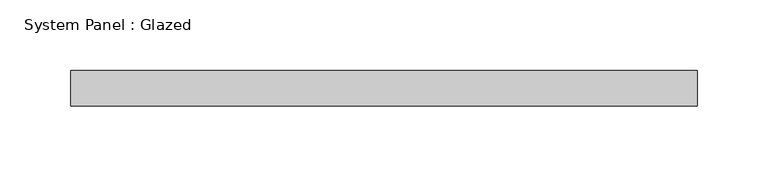
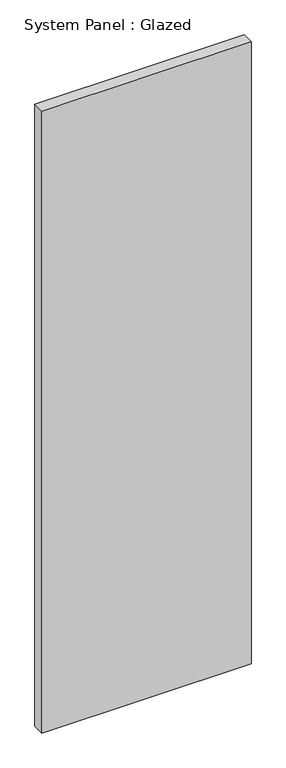
"""IFC4 building model written with IfcOpenShell, lengths in millimetres: plate geometry, System Panel : Glazed."""

from ifc_helpers import new_model, si_unit, origin, origin_with_axes, place, context, project, spatial, polyline, outline, extrude, source, transform, mapped, element, save


def system_panel_glazed_17c4a998(model_context):
    return source(origin(), model_context, "Body", "SweptSolid", [
        extrude(outline(polyline([(222.25, 19.05), (-222.25, 19.05), (-222.25, 44.45), (222.25, 44.45), (222.25, 19.05)])), origin_with_axes(), (0.0, 0.0, 1.0), 1397.0),
    ])


if __name__ == "__main__":
    model = new_model("IFC4")
    model_context = context("Model", 3, world=origin())
    ifc_project = project(units=[si_unit("LENGTHUNIT", "METRE", prefix="MILLI")], contexts=[model_context])
    site = spatial("IfcSite", under=ifc_project)
    building = spatial("IfcBuilding", under=site)
    placement = place(None, origin())
    system_panel_glazed_shape = system_panel_glazed_17c4a998(model_context)
    element("IfcPlate", 1, ObjectType="System Panel : Glazed", at=placement, inside=building, context=model_context, shape_type="MappedRepresentation", body=[
        mapped(system_panel_glazed_shape, transform((0.0, 0.0, 0.0), x_axis=(1.0, 0.0, 0.0), y_axis=(0.0, 1.0, 0.0), z_axis=(0.0, 0.0, 1.0))),
    ])
    save(model, "model.ifc")

# Revit data of these elements
# Type "System Panel : Glazed"
#   Construction Type Id = "GSP4R"
#   Analytic Construction = "1/8 in Pilkington single glazing"
#   Visual Light Transmittance = 0.9
#   Solar Heat Gain Coefficient = 0.86
#   Heat Transfer Coefficient (U) = 1.18115 BTU/(h·ft²·°F)
#   Define Thermal Properties by = 1
# Element 1 (IfcPlate, "System Panel : Glazed")
#   Materials on its faces: "Glass"
# Materials
#   "Glass": class "Glass", colour RGB 0 128 192, transparency 0.75, Description = "Soda Lime Glass", Cost = 0
